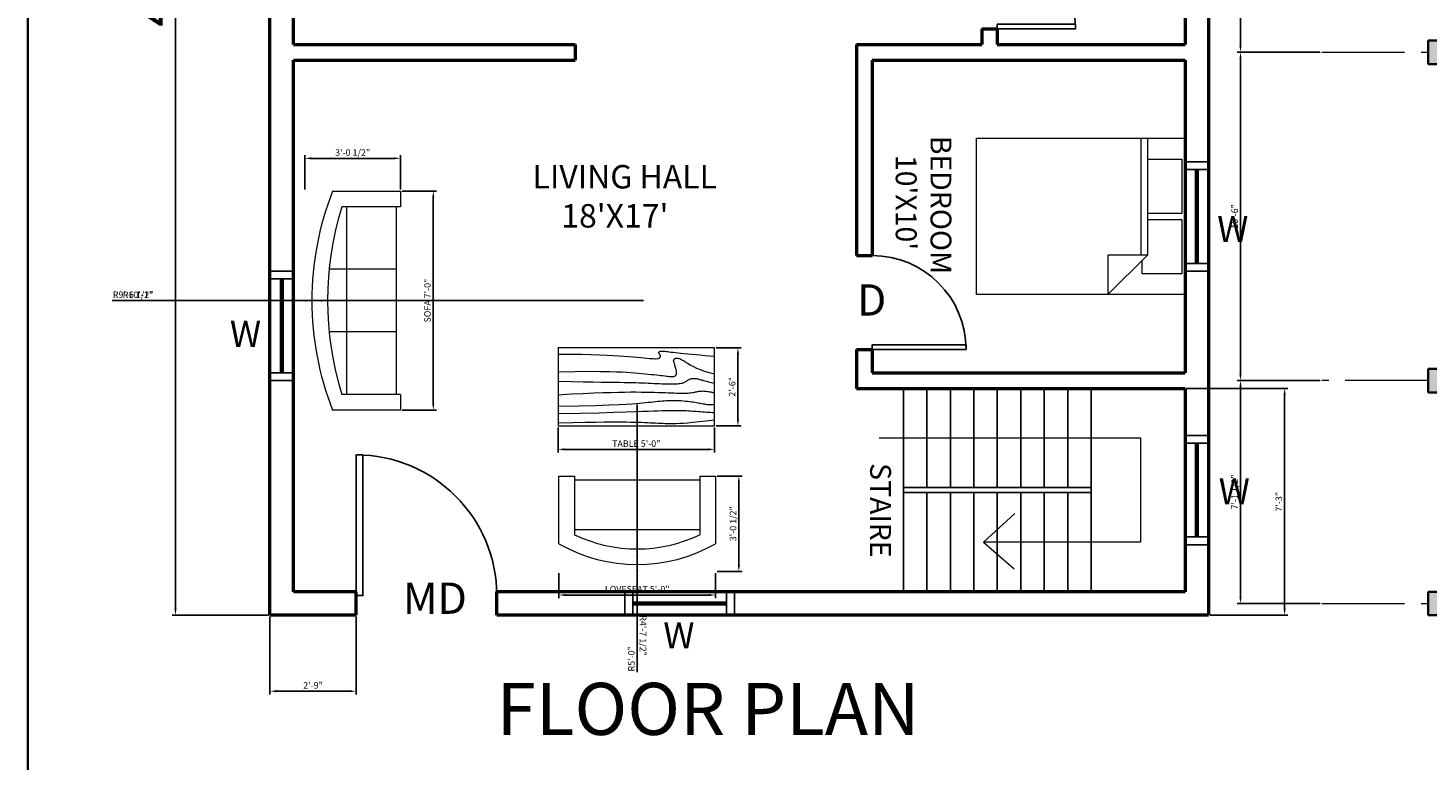
# Model space of a CAD drawing. Units: inches. Extents: x 2150 to 10686, y 1035 to 5077.
# Tile 2 of 12: x 2150 to 2687, y 1472 to 1753. Entities that reach past the tile are written whole.
import ezdxf

# ---------------------------------------------------------------- set-up
doc = ezdxf.new("R2010")
doc.units = ezdxf.units.IN
doc.linetypes.add('CENTER', pattern=[50.8, 31.75, -6.35, 6.35, -6.35])
for name, color, linetype, lineweight in [('A-ANNO-DIMS', 2, 'Continuous', 18), ('A-ANNO-IDEN', 2, 'Continuous', 18), ('A-ANNO-SYMB', 3, 'Continuous', 18), ('A-ANNO-TITL', 3, 'Continuous', 35), ('A-ANNO-TTLB', 7, 'Continuous', 35), ('A-AREA-IDEN', 7, 'Continuous', 18), ('A-COLS', 7, 'Continuous', 35), ('A-COLS-PATT', 8, 'Continuous', 13), ('A-DOOR', 4, 'Continuous', 25), ('A-FLOR-STRS', 4, 'Continuous', 25), ('A-FURN', 8, 'Continuous', 18), ('A-GLAZ', 30, 'Continuous', 25), ('A-GRID', 1, 'CENTER', 18), ('A-WALL', 18, 'Continuous', 50)]:
    doc.layers.add(name, color=color, linetype=linetype, lineweight=lineweight)
doc.styles.get("Standard").update_dxf_attribs({"font": 'arial.ttf'})
doc.dimstyles.new('ISO-25', dxfattribs={"dimtxt": 2.5, "dimasz": 2.5, "dimexe": 1.25, "dimexo": 0.625, "dimtad": 1, "dimdec": 0, "dimlunit": 3, "dimtxsty": 'Standard', "dimcen": 2.5, "dimadec": 0, "dimazin": 0, "dimtfac": 1, "dimtdec": 0, "dimtmove": 0, "dimatfit": 3, "dimfxl": 1, "dimarcsym": 0})

# ---------------------------------------------------------------- blocks, each defined once
blk = doc.blocks.new('Bed - Queen')
for p, q in [((0, -80.00003), (0, 0)), ((0, 0), (59.99999, 0)), ((59.99999, 0), (59.99999, -80.00003)), ((7.99999, -1.2), (28.79998, -1.2)), ((7.99999, -14.4), (7.99999, -1.2)), ((28.79998, -1.2), (28.79998, -14.4)), ((31.19999, -1.2), (51.99999, -1.2)), ((31.19999, -14.4), (31.19999, -1.2)), ((51.99999, -1.2), (51.99999, -16.4)), ((0, -14.4), (44.8, -14.4)), ((59.99999, -29.6), (44.8, -14.4)), ((44.8, -14.4), (44.8, -29.6)), ((44.8, -16.8), (0, -16.8)), ((51.99999, -16.4), (46.79936, -16.4)), ((44.8, -29.6), (59.99999, -29.6)), ((59.99999, -80.00003), (0, -80.00003))]:
    blk.add_line(p, q)
blk = doc.blocks.new('Sofa - Roundback 7 ft.')
for p, q in [((-12.00002, -32.4421), (-12.00003, -6.5971)), ((11.99997, -32.4421), (11.99998, -6.5971)), ((-36.000027, -34), (-36.000027, -11.4696)), ((-35.999844, -13.3819), (35.9998, -13.3819)), ((35.99998, -34), (35.99998, -11.4696)), ((-36.000027, -32.4421), (35.99998, -32.4421))]:
    blk.add_line(p, q)
for points in [[(-36.000027, -34), (-42.000027, -34), (-42.000027, -8)], [(41.99998, -8), (41.99998, -34), (35.99998, -34)]]:
    blk.add_lwpolyline(points)
for centre, radius, start, end in [((0, -114.25), 114.25, 68.43141, 111.5686), ((-0.00001, -127.1968), 121.1968, 72.72033, 107.2797)]:
    blk.add_arc(centre, radius, start, end)
blk = doc.blocks.new('Sofa - Roundback Loveseat 5 ft.')
for p, q in [((0, -32.44198), (0, -5.99998)), ((-24, -33.99998), (-24, -11.46958)), ((-23.9998, -13.38178), (23.99986, -13.38178)), ((24.00004, -33.99998), (24.00004, -11.46958)), ((-24, -32.44198), (24.00004, -32.44198))]:
    blk.add_line(p, q)
for points in [[(-24, -33.99998), (-30, -33.99998), (-30, -7.99998)], [(30.00004, -7.99998), (30.00004, -33.99998), (24.00004, -33.99998)]]:
    blk.add_lwpolyline(points)
for centre, radius, start, end in [((0, -60.24998), 60.24998, 60.13715, 119.8628), ((0, -61.38438), 55.38444, 64.32083, 115.6792)]:
    blk.add_arc(centre, radius, start, end)
blk = doc.blocks.new('Table - Rectangular Woodgrain 60 x 30 in.')
for p, q in [((0, 0), (0, -30)), ((60, 0), (0, 0)), ((60, -30), (60, 0)), ((0, -30), (60, -30))]:
    blk.add_line(p, q)
for points in [[(0, -2.4), (4.8155, -2.418), (9.0302, -2.4688), (12.709, -2.5477), (15.9167, -2.65), (18.7181, -2.7711), (21.1781, -2.9063), (23.3616, -3.0508), (25.3333, -3.2), (27.1477, -3.3495), (28.8172, -3.4958), (30.3437, -3.636), (31.7291, -3.7667), (32.9756, -3.8849), (34.0849, -3.9875), (35.059, -4.0714), (35.9, -4.1334), (36.6114, -4.1711), (37.2041, -4.1854), (37.6906, -4.1779), (38.0833, -4.15), (38.3948, -4.1034), (38.6375, -4.0396), (38.8239, -3.9602), (38.9666, -3.8667), (39.0764, -3.7608), (39.1573, -3.6448), (39.2116, -3.521), (39.2416, -3.3917), (39.2498, -3.2593), (39.2385, -3.1261), (39.21, -2.9944), (39.1666, -2.8667), (39.111, -2.7447), (39.0468, -2.6281), (38.978, -2.5163), (38.9083, -2.4083), (38.8418, -2.3035), (38.7823, -2.201), (38.7337, -2.1001), (38.7, -2), (38.6844, -1.9003), (38.6875, -1.8021), (38.7094, -1.707), (38.75, -1.6167), (38.8094, -1.5326), (38.8875, -1.4563), (38.9844, -1.3893), (39.1, -1.3333), (39.2351, -1.2896), (39.3937, -1.2583), (39.5804, -1.2396), (39.8, -1.2333), (40.057, -1.2396), (40.3562, -1.2583), (40.7023, -1.2896), (41.1, -1.3333), (41.5547, -1.3895), (42.0755, -1.4573), (42.6721, -1.5361), (43.3542, -1.625), (44.1316, -1.7233), (45.014, -1.8302), (46.0114, -1.9449), (47.1333, -2.0667), (48.3862, -2.1947), (49.7625, -2.3281), (51.2513, -2.4663), (52.8416, -2.6083), (54.5226, -2.7535), (56.2833, -2.9011), (58.1127, -3.0501), (60, -3.2)], [(0, -9.2), (6.5759, -9.0858), (11.9385, -9.0365), (16.2527, -9.0418), (19.6833, -9.0917), (22.3952, -9.1759), (24.5531, -9.2844), (26.322, -9.4069), (27.8666, -9.5333), (29.3241, -9.6553), (30.7203, -9.7719), (32.0532, -9.8837), (33.3208, -9.9917), (34.5213, -10.0965), (35.6526, -10.199), (36.7128, -10.2999), (37.7, -10.4), (38.6129, -10.4996), (39.4531, -10.5969), (40.223, -10.6895), (40.925, -10.775), (41.5613, -10.8512), (42.1344, -10.9156), (42.6465, -10.966), (43.1, -11), (43.4976, -11.0158), (43.8437, -11.0136), (44.143, -10.9942), (44.4, -10.9583), (44.6195, -10.9069), (44.8062, -10.8406), (44.9648, -10.7603), (45.1, -10.6667), (45.2155, -10.5598), (45.3114, -10.4365), (45.3871, -10.2929), (45.4416, -10.125), (45.4743, -9.929), (45.4844, -9.7011), (45.4709, -9.4371), (45.4333, -9.1333), (45.3716, -8.7883), (45.2896, -8.4104), (45.1919, -8.0107), (45.0833, -7.6), (44.9685, -7.1893), (44.8521, -6.7896), (44.7388, -6.4117), (44.6333, -6.0667), (44.54, -5.7628), (44.4614, -5.4979), (44.4001, -5.2675), (44.3583, -5.0667), (44.3384, -4.8909), (44.3427, -4.7354), (44.3736, -4.5956), (44.4333, -4.4667), (44.5236, -4.3453), (44.6427, -4.2333), (44.7884, -4.1339), (44.9583, -4.05), (45.1501, -3.9849), (45.3614, -3.9417), (45.59, -3.9234), (45.8333, -3.9333), (46.0915, -3.9749), (46.3734, -4.0531), (46.6906, -4.1736), (47.0542, -4.3417), (47.4756, -4.5629), (47.9661, -4.8427), (48.5372, -5.1866), (49.2, -5.6), (49.9676, -6.0844), (50.8594, -6.625), (51.8965, -7.2031), (53.1, -7.8), (54.491, -8.3969), (56.0906, -8.975), (57.9199, -9.5156), (60, -10)], [(0, -12.8), (5.1847, -12.9322), (9.6213, -13.0323), (13.3963, -13.1059), (16.5958, -13.1583), (19.3063, -13.1952), (21.614, -13.2219), (23.6054, -13.2439), (25.3666, -13.2667), (26.9728, -13.2947), (28.4531, -13.3281), (29.8256, -13.3663), (31.1083, -13.4083), (32.3191, -13.4535), (33.476, -13.501), (34.597, -13.5501), (35.7, -13.6), (36.7984, -13.6497), (37.8875, -13.6979), (38.9578, -13.743), (40, -13.7833), (41.0047, -13.8174), (41.9625, -13.8438), (42.864, -13.8607), (43.7, -13.8667), (44.4631, -13.8604), (45.1552, -13.8417), (45.7801, -13.8104), (46.3416, -13.7667), (46.8439, -13.7104), (47.2906, -13.6417), (47.6858, -13.5604), (48.0333, -13.4667), (48.3375, -13.3608), (48.6042, -13.2448), (48.8396, -13.121), (49.05, -12.9917), (49.2417, -12.8593), (49.4208, -12.7261), (49.5937, -12.5944), (49.7667, -12.4667), (49.9452, -12.3451), (50.1323, -12.2313), (50.3303, -12.1268), (50.5416, -12.0333), (50.7686, -11.9524), (51.0135, -11.8854), (51.2788, -11.8341), (51.5666, -11.8), (51.8785, -11.7843), (52.2116, -11.7865), (52.562, -11.8059), (52.926, -11.8417), (53.2998, -11.8931), (53.6795, -11.9594), (54.0614, -12.0397), (54.4416, -12.1333), (54.8223, -12.2401), (55.2293, -12.3625), (55.6942, -12.5037), (56.2489, -12.6667), (56.9251, -12.8547), (57.7545, -13.0708), (58.7689, -13.3182), (60, -13.6)], [(0, -18), (5.124, -17.7273), (9.6609, -17.5057), (13.6705, -17.3303), (17.2125, -17.1958), (20.3467, -17.0973), (23.1328, -17.0297), (25.6307, -16.9878), (27.9, -16.9667), (29.9928, -16.9617), (31.9302, -16.9703), (33.7254, -16.9907), (35.3917, -17.0208), (36.9423, -17.0588), (38.3906, -17.1026), (39.7499, -17.1503), (41.0333, -17.2), (42.2519, -17.2496), (43.4073, -17.2969), (44.4986, -17.3395), (45.525, -17.375), (46.4858, -17.4012), (47.3802, -17.4156), (48.2074, -17.416), (48.9667, -17.4), (49.6583, -17.3662), (50.2872, -17.3167), (50.8595, -17.2547), (51.3812, -17.1833), (51.8584, -17.1057), (52.2971, -17.025), (52.7034, -16.9443), (53.0833, -16.8667), (53.443, -16.7951), (53.789, -16.7313), (54.128, -16.6768), (54.4666, -16.6334), (54.8115, -16.6024), (55.1693, -16.5854), (55.5465, -16.5841), (55.95, -16.6), (56.3828, -16.6337), (56.8346, -16.6823), (57.2915, -16.7418), (57.7396, -16.8084), (58.165, -16.878), (58.5539, -16.9469), (58.8924, -17.0111), (59.1666, -17.0667), (59.3679, -17.1107), (59.5078, -17.1438), (59.6032, -17.1675), (59.6708, -17.1833), (59.7275, -17.193), (59.7901, -17.1979), (59.8753, -17.1998), (60, -17.2)], [(0, -22.4), (8.0098, -22.2501), (14.4094, -22.1011), (19.4168, -21.9535), (23.25, -21.8083), (26.1269, -21.6663), (28.2656, -21.5281), (29.884, -21.3947), (31.2, -21.2667), (32.3967, -21.1448), (33.5172, -21.0292), (34.5697, -20.9198), (35.5625, -20.8167), (36.5037, -20.7198), (37.4015, -20.6292), (38.2642, -20.5448), (39.1, -20.4667), (39.9164, -20.3951), (40.7187, -20.3313), (41.5117, -20.2768), (42.3, -20.2333), (43.0883, -20.2024), (43.8812, -20.1854), (44.6836, -20.1841), (45.5, -20.2), (46.3328, -20.234), (47.1747, -20.2844), (48.0163, -20.3488), (48.8479, -20.425), (49.66, -20.5106), (50.4429, -20.6031), (51.1872, -20.7004), (51.8833, -20.8), (52.5246, -20.8999), (53.1166, -20.9995), (53.6681, -21.0983), (54.1875, -21.1958), (54.6834, -21.2919), (55.1646, -21.3859), (55.6394, -21.4777), (56.1167, -21.5667), (56.6028, -21.6515), (57.0961, -21.7266), (57.5929, -21.7852), (58.0896, -21.8208), (58.5823, -21.8268), (59.0674, -21.7964), (59.5412, -21.723), (60, -21.6)], [(0, -25.2), (8.6355, -25.0504), (15.7026, -24.9031), (21.4049, -24.7606), (25.9458, -24.625), (29.529, -24.4988), (32.3578, -24.3844), (34.6359, -24.284), (36.5667, -24.2), (38.3213, -24.1341), (39.9417, -24.0854), (41.437, -24.0523), (42.8167, -24.0333), (44.0901, -24.0268), (45.2667, -24.0313), (46.3557, -24.0451), (47.3667, -24.0667), (48.309, -24.0947), (49.1928, -24.1287), (50.0284, -24.168), (50.826, -24.2125), (51.5959, -24.2617), (52.3483, -24.3151), (53.0935, -24.3725), (53.8417, -24.4334), (54.6009, -24.497), (55.3699, -24.561), (56.1454, -24.6226), (56.9239, -24.6792), (57.7021, -24.7279), (58.4764, -24.7662), (59.2435, -24.7911), (60, -24.8)], [(0, -28.8), (5.6867, -28.6681), (10.45, -28.5698), (14.407, -28.5012), (17.675, -28.4584), (20.3711, -28.4374), (22.6125, -28.4344), (24.5164, -28.4455), (26.2, -28.4667), (27.762, -28.4947), (29.2276, -28.5281), (30.6033, -28.5663), (31.8958, -28.6084), (33.1118, -28.6535), (34.2578, -28.7011), (35.3405, -28.7501), (36.3666, -28.8), (37.3443, -28.8497), (38.288, -28.8974), (39.2137, -28.9412), (40.1375, -28.9792), (41.0753, -29.0093), (42.0432, -29.0297), (43.0572, -29.0384), (44.1333, -29.0333), (45.2936, -29.0114), (46.5843, -28.9641), (48.0579, -28.8816), (49.7666, -28.7542), (51.7629, -28.5721), (54.0989, -28.3255), (56.8272, -28.0048), (60, -27.6)]]:
    blk.add_lwpolyline(points)
blk = doc.blocks.new('*U9')
for p, q in [((0, 0), (0, -6)), ((-36, 0), (-36, -6))]:
    blk.add_line(p, q)
blk.add_lwpolyline([(0, 0), (0, 36), (-1.75, 36), (-1.75, 0)], close=True)
blk.add_arc((0, 0), 36, 90, 180)
blk = doc.blocks.new('*U10')
for p, q in [((-30, 0), (-30, -6)), ((0, 0), (0, -6))]:
    blk.add_line(p, q)
blk.add_lwpolyline([(0, 0), (0, 30), (-1.75, 30), (-1.75, 0)], close=True)
blk.add_arc((0, 0), 30, 90, 180)
blk = doc.blocks.new('*U11')
for p, q in [((0, 0), (0, -5)), ((36, 0), (36, -5))]:
    blk.add_line(p, q)
blk.add_lwpolyline([(0, 0), (0, 36), (1.75, 36), (1.75, 0)], close=True)
blk.add_arc((0, 0), 36, 0, 90)
blk = doc.blocks.new('*D13')
at = {"layer": 'A-ANNO-DIMS', "color": 0, "lineweight": -2, "transparency": 16777216}
for p, q in [((2242.07, 2007.29), (2205.18, 2007.29)), ((2206.43, 2004.79), (2206.43, 1529.79)), ((2242.07, 1527.29), (2205.18, 1527.29))]:
    blk.add_line(p, q, dxfattribs=at)
at = {"layer": 'A-ANNO-DIMS', "color": 0, "transparency": 16777216}
for points in [[(2206.01, 2004.79), (2206.85, 2004.79), (2206.43, 2007.29)], [(2206.01, 1529.79), (2206.85, 1529.79), (2206.43, 1527.29)]]:
    blk.add_solid(points, dxfattribs=at)
at = {"layer": 'Defpoints', "color": 0, "transparency": 16777216}
for p in [(2242.69, 2007.29), (2206.43, 1527.29), (2242.69, 1527.29)]:
    blk.add_point(p, dxfattribs=at)
at = {"layer": 'A-ANNO-DIMS', "color": 0, "transparency": 16777216, "insert": (2198.15, 1767.29), "char_height": 2.5, "attachment_point": 5, "rotation": 90}
blk.add_mtext("{\\H6x;40'}", dxfattribs=at)
blk = doc.blocks.new('COL-SQUARE-9IN')
for p, q in [((0, 9), (9, 9)), ((0, 0), (0, 9)), ((9, 9), (9, 0)), ((9, 0), (0, 0))]:
    blk.add_line(p, q)
blk = doc.blocks.new('WINDOW-36IN')
for p, q in [((9, 42), (0, 42)), ((9, 39), (0, 39)), ((4, 39), (4, 3)), ((4.5, 39), (4.5, 3)), ((5, 39), (5, 3)), ((9, 3), (0, 3)), ((9, 0), (0, 0))]:
    blk.add_line(p, q)
blk = doc.blocks.new('*D48')
at = {"layer": 'A-ANNO-DIMS', "color": 0, "lineweight": -2, "transparency": 16777216}
for p, q in [((2293.35, 1690), (2306.58, 1690)), ((2305.33, 1608.5), (2305.33, 1687.5)), ((2293.35, 1606), (2306.58, 1606))]:
    blk.add_line(p, q, dxfattribs=at)
at = {"layer": 'A-ANNO-DIMS', "color": 0, "transparency": 16777216}
for points in [[(2304.91, 1687.5), (2305.75, 1687.5), (2305.33, 1690)], [(2304.91, 1608.5), (2305.75, 1608.5), (2305.33, 1606)]]:
    blk.add_solid(points, dxfattribs=at)
at = {"layer": 'Defpoints', "color": 0, "transparency": 16777216}
for p in [(2292.73, 1690), (2305.33, 1690), (2292.73, 1606)]:
    blk.add_point(p, dxfattribs=at)
at = {"layer": 'A-ANNO-DIMS', "color": 0, "transparency": 16777216, "insert": (2303.41, 1648), "char_height": 2.5, "attachment_point": 5, "rotation": 90}
blk.add_mtext('SOFA 7\'-0"', dxfattribs=at)
blk = doc.blocks.new('*D49')
at = {"layer": 'A-ANNO-DIMS', "color": 0, "lineweight": -2, "transparency": 16777216}
for p, q in [((2256.06, 1690.62), (2256.06, 1703.85)), ((2290.23, 1702.6), (2258.56, 1702.6)), ((2292.73, 1690.62), (2292.73, 1703.85))]:
    blk.add_line(p, q, dxfattribs=at)
at = {"layer": 'A-ANNO-DIMS', "color": 0, "transparency": 16777216}
for points in [[(2258.56, 1703.01), (2258.56, 1702.18), (2256.06, 1702.6)], [(2290.23, 1703.01), (2290.23, 1702.18), (2292.73, 1702.6)]]:
    blk.add_solid(points, dxfattribs=at)
at = {"layer": 'Defpoints', "color": 0, "transparency": 16777216}
for p in [(2256.06, 1702.6), (2256.06, 1690), (2292.73, 1690)]:
    blk.add_point(p, dxfattribs=at)
at = {"layer": 'A-ANNO-DIMS', "color": 0, "transparency": 16777216, "insert": (2274.4, 1704.52), "char_height": 2.5, "attachment_point": 5}
blk.add_mtext('3\'-0 1/2"', dxfattribs=at)
blk = doc.blocks.new('*D52')
at = {"layer": 'A-ANNO-DIMS', "color": 0, "lineweight": -2, "transparency": 16777216}
for p, q in [((2353.54, 1543.39), (2353.54, 1533.76)), ((2413.54, 1543.39), (2413.54, 1533.76)), ((2411.04, 1535.01), (2356.04, 1535.01))]:
    blk.add_line(p, q, dxfattribs=at)
at = {"layer": 'A-ANNO-DIMS', "color": 0, "transparency": 16777216}
for points in [[(2356.04, 1535.43), (2356.04, 1534.6), (2353.54, 1535.01)], [(2411.04, 1535.43), (2411.04, 1534.6), (2413.54, 1535.01)]]:
    blk.add_solid(points, dxfattribs=at)
at = {"layer": 'Defpoints', "color": 0, "transparency": 16777216}
for p in [(2353.54, 1544.01), (2413.54, 1544.01), (2353.54, 1535.01)]:
    blk.add_point(p, dxfattribs=at)
at = {"layer": 'A-ANNO-DIMS', "color": 0, "transparency": 16777216, "insert": (2383.54, 1536.93), "char_height": 2.5, "attachment_point": 5}
blk.add_mtext('LOVESEAT 5\'-0"', dxfattribs=at)
blk = doc.blocks.new('*D53')
at = {"layer": 'A-ANNO-DIMS', "color": 0, "lineweight": -2, "transparency": 16777216}
for p, q in [((2414.17, 1580.68), (2423.79, 1580.68)), ((2422.54, 1578.18), (2422.54, 1546.51)), ((2414.17, 1544.01), (2423.79, 1544.01))]:
    blk.add_line(p, q, dxfattribs=at)
at = {"layer": 'A-ANNO-DIMS', "color": 0, "transparency": 16777216}
for points in [[(2422.13, 1578.18), (2422.96, 1578.18), (2422.54, 1580.68)], [(2422.13, 1546.51), (2422.96, 1546.51), (2422.54, 1544.01)]]:
    blk.add_solid(points, dxfattribs=at)
at = {"layer": 'Defpoints', "color": 0, "transparency": 16777216}
for p in [(2413.54, 1580.68), (2413.54, 1544.01), (2422.54, 1544.01)]:
    blk.add_point(p, dxfattribs=at)
at = {"layer": 'A-ANNO-DIMS', "color": 0, "transparency": 16777216, "insert": (2420.63, 1562.35), "char_height": 2.5, "attachment_point": 5, "rotation": 90}
blk.add_mtext('3\'-0 1/2"', dxfattribs=at)
blk = doc.blocks.new('*D60')
at = {"layer": 'A-ANNO-DIMS', "color": 0, "lineweight": -2, "transparency": 16777216}
for p, q in [((2353.19, 1599.26), (2353.19, 1589.64)), ((2413.19, 1599.26), (2413.19, 1589.64)), ((2355.69, 1590.89), (2410.69, 1590.89))]:
    blk.add_line(p, q, dxfattribs=at)
at = {"layer": 'A-ANNO-DIMS', "color": 0, "transparency": 16777216}
for points in [[(2355.69, 1591.31), (2355.69, 1590.47), (2353.19, 1590.89)], [(2410.69, 1591.31), (2410.69, 1590.47), (2413.19, 1590.89)]]:
    blk.add_solid(points, dxfattribs=at)
at = {"layer": 'Defpoints', "color": 0, "transparency": 16777216}
for p in [(2353.19, 1599.89), (2413.19, 1599.89), (2413.19, 1590.89)]:
    blk.add_point(p, dxfattribs=at)
at = {"layer": 'A-ANNO-DIMS', "color": 0, "transparency": 16777216, "insert": (2383.19, 1592.79), "char_height": 2.5, "attachment_point": 5}
blk.add_mtext('TABLE 5\'-0"', dxfattribs=at)
blk = doc.blocks.new('*D61')
at = {"layer": 'A-ANNO-DIMS', "color": 0, "lineweight": -2, "transparency": 16777216}
for p, q in [((2413.81, 1629.89), (2423.44, 1629.89)), ((2422.19, 1602.39), (2422.19, 1627.39)), ((2413.81, 1599.89), (2423.44, 1599.89))]:
    blk.add_line(p, q, dxfattribs=at)
at = {"layer": 'A-ANNO-DIMS', "color": 0, "transparency": 16777216}
for points in [[(2421.77, 1627.39), (2422.6, 1627.39), (2422.19, 1629.89)], [(2421.77, 1602.39), (2422.6, 1602.39), (2422.19, 1599.89)]]:
    blk.add_solid(points, dxfattribs=at)
at = {"layer": 'Defpoints', "color": 0, "transparency": 16777216}
for p in [(2413.19, 1629.89), (2422.19, 1629.89), (2413.19, 1599.89)]:
    blk.add_point(p, dxfattribs=at)
at = {"layer": 'A-ANNO-DIMS', "color": 0, "transparency": 16777216, "insert": (2420.29, 1614.89), "char_height": 2.5, "attachment_point": 5, "rotation": 90}
blk.add_mtext('2\'-6"', dxfattribs=at)
blk = doc.blocks.new('*D81')
at = {"layer": 'A-ANNO-DIMS', "color": 0, "lineweight": -2, "transparency": 16777216}
for p, q in [((2645.54, 1869.29), (2613.71, 1869.29)), ((2614.96, 1866.79), (2614.96, 1745.79)), ((2645.54, 1743.29), (2613.71, 1743.29))]:
    blk.add_line(p, q, dxfattribs=at)
at = {"layer": 'A-ANNO-DIMS', "color": 0, "transparency": 16777216}
for points in [[(2614.55, 1866.79), (2615.38, 1866.79), (2614.96, 1869.29)], [(2614.55, 1745.79), (2615.38, 1745.79), (2614.96, 1743.29)]]:
    blk.add_solid(points, dxfattribs=at)
at = {"layer": 'Defpoints', "color": 0, "transparency": 16777216}
for p in [(2646.16, 1869.29), (2614.96, 1743.29), (2646.16, 1743.29)]:
    blk.add_point(p, dxfattribs=at)
at = {"layer": 'A-ANNO-DIMS', "color": 0, "transparency": 16777216, "insert": (2613.06, 1806.29), "char_height": 2.5, "attachment_point": 5, "rotation": 90}
blk.add_mtext('10\'-6"', dxfattribs=at)
blk = doc.blocks.new('*D82')
at = {"layer": 'A-ANNO-DIMS', "color": 0, "lineweight": -2, "transparency": 16777216}
for p, q in [((2645.54, 1743.29), (2613.71, 1743.29)), ((2614.96, 1740.79), (2614.96, 1619.79)), ((2645.54, 1617.29), (2613.71, 1617.29))]:
    blk.add_line(p, q, dxfattribs=at)
at = {"layer": 'A-ANNO-DIMS', "color": 0, "transparency": 16777216}
for points in [[(2614.55, 1740.79), (2615.38, 1740.79), (2614.96, 1743.29)], [(2614.55, 1619.79), (2615.38, 1619.79), (2614.96, 1617.29)]]:
    blk.add_solid(points, dxfattribs=at)
at = {"layer": 'Defpoints', "color": 0, "transparency": 16777216}
for p in [(2646.16, 1743.29), (2614.96, 1617.29), (2646.16, 1617.29)]:
    blk.add_point(p, dxfattribs=at)
at = {"layer": 'A-ANNO-DIMS', "color": 0, "transparency": 16777216, "insert": (2613.06, 1680.29), "char_height": 2.5, "attachment_point": 5, "rotation": 90}
blk.add_mtext('10\'-6"', dxfattribs=at)
blk = doc.blocks.new('*D83')
at = {"layer": 'A-ANNO-DIMS', "color": 0, "lineweight": -2, "transparency": 16777216}
for p, q in [((2645.54, 1617.29), (2613.71, 1617.29)), ((2614.96, 1614.79), (2614.96, 1534.29)), ((2645.54, 1531.79), (2613.71, 1531.79))]:
    blk.add_line(p, q, dxfattribs=at)
at = {"layer": 'A-ANNO-DIMS', "color": 0, "transparency": 16777216}
for points in [[(2614.55, 1614.79), (2615.38, 1614.79), (2614.96, 1617.29)], [(2614.55, 1534.29), (2615.38, 1534.29), (2614.96, 1531.79)]]:
    blk.add_solid(points, dxfattribs=at)
at = {"layer": 'Defpoints', "color": 0, "transparency": 16777216}
for p in [(2646.16, 1617.29), (2614.96, 1531.79), (2646.16, 1531.79)]:
    blk.add_point(p, dxfattribs=at)
at = {"layer": 'A-ANNO-DIMS', "color": 0, "transparency": 16777216, "insert": (2613.05, 1574.54), "char_height": 2.5, "attachment_point": 5, "rotation": 90}
blk.add_mtext('7\'-1 1/2"', dxfattribs=at)
blk = doc.blocks.new('*D139')
at = {"layer": 'A-ANNO-DIMS', "color": 0, "lineweight": -2, "transparency": 16777216}
for p, q in [((2242.69, 1526.67), (2242.69, 1496.84)), ((2275.69, 1526.67), (2275.69, 1496.84)), ((2245.19, 1498.09), (2273.19, 1498.09))]:
    blk.add_line(p, q, dxfattribs=at)
at = {"layer": 'A-ANNO-DIMS', "color": 0, "transparency": 16777216}
for points in [[(2245.19, 1498.51), (2245.19, 1497.67), (2242.69, 1498.09)], [(2273.19, 1498.51), (2273.19, 1497.67), (2275.69, 1498.09)]]:
    blk.add_solid(points, dxfattribs=at)
at = {"layer": 'Defpoints', "color": 0, "transparency": 16777216}
for p in [(2242.69, 1527.29), (2275.69, 1527.29), (2275.69, 1498.09)]:
    blk.add_point(p, dxfattribs=at)
at = {"layer": 'A-ANNO-DIMS', "color": 0, "transparency": 16777216, "insert": (2259.19, 1499.99), "char_height": 2.5, "attachment_point": 5}
blk.add_mtext('2\'-9"', dxfattribs=at)
blk = doc.blocks.new('*D140')
at = {"layer": 'A-ANNO-DIMS', "color": 0, "lineweight": -2, "transparency": 16777216}
for p, q in [((2594.32, 1614.29), (2633.14, 1614.29)), ((2631.89, 1529.79), (2631.89, 1611.79)), ((2603.32, 1527.29), (2633.14, 1527.29))]:
    blk.add_line(p, q, dxfattribs=at)
at = {"layer": 'A-ANNO-DIMS', "color": 0, "transparency": 16777216}
for points in [[(2631.48, 1611.79), (2632.31, 1611.79), (2631.89, 1614.29)], [(2631.48, 1529.79), (2632.31, 1529.79), (2631.89, 1527.29)]]:
    blk.add_solid(points, dxfattribs=at)
at = {"layer": 'Defpoints', "color": 0, "transparency": 16777216}
for p in [(2593.69, 1614.29), (2631.89, 1614.29), (2602.69, 1527.29)]:
    blk.add_point(p, dxfattribs=at)
at = {"layer": 'A-ANNO-DIMS', "color": 0, "transparency": 16777216, "insert": (2629.99, 1570.79), "char_height": 2.5, "attachment_point": 5, "rotation": 90}
blk.add_mtext('7\'-3"', dxfattribs=at)
blk = doc.blocks.new('*D147')
at = {"layer": 'A-ANNO-DIMS', "color": 0, "lineweight": -2, "transparency": 16777216}
for p, q in [((2185.9, 1648), (2262.23, 1648)), ((2385.93, 1648), (2264.73, 1648))]:
    blk.add_line(p, q, dxfattribs=at)
at = {"layer": 'A-ANNO-DIMS', "color": 0, "transparency": 16777216}
blk.add_solid([(2262.23, 1648.41), (2262.23, 1647.58), (2264.73, 1648)], dxfattribs=at)
at = {"layer": 'Defpoints', "color": 0, "transparency": 16777216}
for p in [(2264.73, 1648), (2385.93, 1648)]:
    blk.add_point(p, dxfattribs=at)
at = {"layer": 'A-ANNO-DIMS', "color": 0, "transparency": 16777216, "insert": (2192.01, 1649.9), "char_height": 2.5, "attachment_point": 5, "rotation": 0.0001}
blk.add_mtext('R10\'-1"', dxfattribs=at)
blk = doc.blocks.new('*D148')
at = {"layer": 'A-ANNO-DIMS', "color": 0, "lineweight": -2, "transparency": 16777216}
for p, q in [((2182.12, 1648), (2256.23, 1648)), ((2372.98, 1648), (2258.73, 1648))]:
    blk.add_line(p, q, dxfattribs=at)
at = {"layer": 'A-ANNO-DIMS', "color": 0, "transparency": 16777216}
blk.add_solid([(2256.23, 1648.41), (2256.23, 1647.58), (2258.73, 1648)], dxfattribs=at)
at = {"layer": 'Defpoints', "color": 0, "transparency": 16777216}
for p in [(2258.73, 1648), (2372.98, 1648)]:
    blk.add_point(p, dxfattribs=at)
at = {"layer": 'A-ANNO-DIMS', "color": 0, "transparency": 16777216, "insert": (2190.18, 1649.92), "char_height": 2.5, "attachment_point": 5, "rotation": 0.0001}
blk.add_mtext('R9\'-6 1/2"', dxfattribs=at)
blk = doc.blocks.new('*D149')
at = {"layer": 'A-ANNO-DIMS', "color": 0, "lineweight": -2, "transparency": 16777216}
for p, q in [((2383.54, 1606.93), (2383.54, 1546.68)), ((2383.54, 1505.39), (2383.54, 1544.18))]:
    blk.add_line(p, q, dxfattribs=at)
at = {"layer": 'A-ANNO-DIMS', "color": 0, "transparency": 16777216}
blk.add_solid([(2383.13, 1544.18), (2383.96, 1544.18), (2383.54, 1546.68)], dxfattribs=at)
at = {"layer": 'Defpoints', "color": 0, "transparency": 16777216}
for p in [(2383.54, 1606.93), (2383.54, 1546.68)]:
    blk.add_point(p, dxfattribs=at)
at = {"layer": 'A-ANNO-DIMS', "color": 0, "transparency": 16777216, "insert": (2381.64, 1510.53), "char_height": 2.5, "attachment_point": 5, "rotation": 89.9995}
blk.add_mtext('R5\'-0"', dxfattribs=at)
blk = doc.blocks.new('*D150')
at = {"layer": 'A-ANNO-DIMS', "color": 0, "lineweight": -2, "transparency": 16777216}
for p, q in [((2383.54, 1608.06), (2383.54, 1552.68)), ((2383.54, 1511.39), (2383.54, 1550.18))]:
    blk.add_line(p, q, dxfattribs=at)
at = {"layer": 'A-ANNO-DIMS', "color": 0, "transparency": 16777216}
blk.add_solid([(2383.96, 1550.18), (2383.13, 1550.18), (2383.54, 1552.68)], dxfattribs=at)
at = {"layer": 'Defpoints', "color": 0, "transparency": 16777216}
for p in [(2383.54, 1608.06), (2383.54, 1552.68)]:
    blk.add_point(p, dxfattribs=at)
at = {"layer": 'A-ANNO-DIMS', "color": 0, "transparency": 16777216, "insert": (2385.46, 1519.45), "char_height": 2.5, "attachment_point": 5, "rotation": 270.0005}
blk.add_mtext('R4\'-7 1/2"', dxfattribs=at)

msp = doc.modelspace()

# ---------------------------------------------------------------- hatches: boundary and pattern name
at = {"layer": 'A-COLS-PATT'}
h = msp.add_hatch(color=256, dxfattribs=at)
h.dxf.hatch_style = 1
h.paths.add_polyline_path([(2695.9, 2007.29), (2686.9, 2007.29), (2686.9, 1998.29), (2695.9, 1998.29)])
h.paths.add_polyline_path([(2871.4, 2007.29), (2862.4, 2007.29), (2862.4, 1998.29), (2871.4, 1998.29)])
h.paths.add_polyline_path([(3046.9, 2007.29), (3037.9, 2007.29), (3037.9, 1998.29), (3046.9, 1998.29)])
h.paths.add_polyline_path([(2695.9, 1873.79), (2686.9, 1873.79), (2686.9, 1864.79), (2695.9, 1864.79)])
h.paths.add_polyline_path([(2871.4, 1873.79), (2862.4, 1873.79), (2862.4, 1864.79), (2871.4, 1864.79)])
h.paths.add_polyline_path([(3046.9, 1873.79), (3037.9, 1873.79), (3037.9, 1864.79), (3046.9, 1864.79)])
h.paths.add_polyline_path([(2695.9, 1747.79), (2686.9, 1747.79), (2686.9, 1738.79), (2695.9, 1738.79)])
h.paths.add_polyline_path([(2871.4, 1747.79), (2862.4, 1747.79), (2862.4, 1738.79), (2871.4, 1738.79)])
h.paths.add_polyline_path([(3046.9, 1747.79), (3037.9, 1747.79), (3037.9, 1738.79), (3046.9, 1738.79)])
h.paths.add_polyline_path([(2695.9, 1621.79), (2686.9, 1621.79), (2686.9, 1612.79), (2695.9, 1612.79)])
h.paths.add_polyline_path([(2871.4, 1621.79), (2862.4, 1621.79), (2862.4, 1612.79), (2871.4, 1612.79)])
h.paths.add_polyline_path([(3046.9, 1621.79), (3037.9, 1621.79), (3037.9, 1612.79), (3046.9, 1612.79)])
h.paths.add_polyline_path([(2695.9, 1536.29), (2686.9, 1536.29), (2686.9, 1527.29), (2695.9, 1527.29)])
h.paths.add_polyline_path([(2871.4, 1536.29), (2862.4, 1536.29), (2862.4, 1527.29), (2871.4, 1527.29)])
h.paths.add_polyline_path([(3046.9, 1536.29), (3037.9, 1536.29), (3037.9, 1527.29), (3046.9, 1527.29)])

# ---------------------------------------------------------------- linework, layer by layer
at = {"layer": 'A-ANNO-SYMB'}
for p, q in [((2476.32, 1595.29), (2576.67, 1595.29)), ((2576.67, 1595.29), (2576.67, 1555.29)), ((2516.33, 1555.29), (2528.47, 1566.24)), ((2576.67, 1555.29), (2516.33, 1555.29)), ((2516.33, 1555.29), (2528.11, 1545.03))]:
    msp.add_line(p, q, dxfattribs=at)
at = {"layer": 'A-ANNO-TTLB'}
msp.add_lwpolyline([(2149.86, 2100.72), (3159.01, 2100.72), (3159.01, 1034.91), (2149.86, 1034.91)], close=True, dxfattribs=at)
at = {"layer": 'A-FLOR-STRS'}
for p, q in [((2485.69, 1614.29), (2485.69, 1536.29)), ((2494.69, 1614.29), (2494.69, 1576.29)), ((2503.69, 1614.29), (2503.69, 1576.29)), ((2512.69, 1614.29), (2512.69, 1576.29)), ((2521.69, 1614.29), (2521.69, 1576.29)), ((2530.69, 1614.29), (2530.69, 1576.29)), ((2539.69, 1614.29), (2539.69, 1576.29)), ((2548.69, 1614.29), (2548.69, 1576.29)), ((2557.69, 1614.29), (2557.69, 1536.29)), ((2557.69, 1576.29), (2485.69, 1576.29)), ((2557.69, 1574.29), (2485.69, 1574.29)), ((2494.69, 1574.29), (2494.69, 1536.29)), ((2503.69, 1574.29), (2503.69, 1536.29)), ((2512.69, 1574.29), (2512.69, 1536.29)), ((2521.69, 1574.29), (2521.69, 1536.29)), ((2530.69, 1574.29), (2530.69, 1536.29)), ((2539.69, 1574.29), (2539.69, 1536.29)), ((2548.69, 1574.29), (2548.69, 1536.29))]:
    msp.add_line(p, q, dxfattribs=at)
at = {"layer": 'A-GRID'}
for p, q in [((2646.16, 1743.29), (2686.9, 1743.29)), ((2686.9, 1617.29), (2646.16, 1617.29)), ((2646.16, 1531.79), (2686.9, 1531.79))]:
    msp.add_line(p, q, dxfattribs=at)
at = {"layer": 'A-WALL'}
for p, q in [((2242.69, 1527.29), (2242.69, 2007.29)), ((2602.69, 2007.29), (2602.69, 1527.29)), ((2251.69, 1746.29), (2251.69, 1866.29)), ((2593.69, 1818.29), (2593.69, 1746.29)), ((2515.69, 1752.29), (2521.69, 1752.29)), ((2515.69, 1752.29), (2515.69, 1746.29)), ((2521.69, 1752.29), (2521.69, 1746.29)), ((2251.69, 1746.29), (2359.69, 1746.29)), ((2359.69, 1746.29), (2359.69, 1740.29)), ((2467.69, 1746.29), (2515.69, 1746.29)), ((2467.69, 1746.29), (2467.69, 1665.29)), ((2521.69, 1746.29), (2593.69, 1746.29)), ((2251.69, 1536.29), (2251.69, 1740.29)), ((2251.69, 1740.29), (2359.69, 1740.29)), ((2473.69, 1740.29), (2593.69, 1740.29)), ((2473.69, 1740.29), (2473.69, 1665.29)), ((2593.69, 1740.29), (2593.69, 1620.29)), ((2467.69, 1665.29), (2473.69, 1665.29)), ((2467.69, 1629.29), (2473.69, 1629.29)), ((2467.69, 1629.29), (2467.69, 1614.29)), ((2473.69, 1629.29), (2473.69, 1620.29)), ((2473.69, 1620.29), (2593.69, 1620.29)), ((2467.69, 1614.29), (2593.69, 1614.29)), ((2593.69, 1614.29), (2593.69, 1536.29)), ((2275.69, 1536.29), (2251.69, 1536.29)), ((2275.69, 1527.29), (2275.69, 1536.29)), ((2593.69, 1536.29), (2329.69, 1536.29)), ((2329.69, 1527.29), (2329.69, 1536.29)), ((2275.69, 1527.29), (2242.69, 1527.29)), ((2602.69, 1527.29), (2329.69, 1527.29))]:
    msp.add_line(p, q, dxfattribs=at)

# ---------------------------------------------------------------- block references
at = {"layer": 'A-COLS'}
for p in [(2686.9, 1738.79), (2686.9, 1612.79), (2686.9, 1527.29)]:
    msp.add_blockref('COL-SQUARE-9IN', p, dxfattribs=at)
at = {"layer": 'A-DOOR', "rotation": 270}
for name, p in [('*U10', (2521.69, 1752.29)), ('*U9', (2473.69, 1629.29))]:
    msp.add_blockref(name, p, dxfattribs=at)
at = {"layer": 'A-DOOR', "xscale": 1.5, "yscale": 1.5, "zscale": 1.5}
msp.add_blockref('*U11', (2275.69, 1534.79), dxfattribs=at)
at = {"layer": 'A-FURN'}
for name, p, rotation in [('Bed - Queen', (2593.69, 1710.29), 270), ('Sofa - Roundback 7 ft.', (2258.73, 1648), 90), ('Sofa - Roundback Loveseat 5 ft.', (2383.54, 1546.68), 180)]:
    msp.add_blockref(name, p, dxfattribs=dict(at, rotation=rotation))
msp.add_blockref('Table - Rectangular Woodgrain 60 x 30 in.', (2353.19, 1629.89), dxfattribs=at)
at = {"layer": 'A-GLAZ'}
for p in [(2593.69, 1659.29), (2242.69, 1617.29)]:
    msp.add_blockref('WINDOW-36IN', p, dxfattribs=at)
for p, rotation in [((2602.69, 1596.29), 180), ((2420.82, 1527.29), 89.99999999999767)]:
    msp.add_blockref('WINDOW-36IN', p, dxfattribs=dict(at, rotation=rotation))

# ---------------------------------------------------------------- texts
at = {"layer": 'A-ANNO-IDEN', "attachment_point": 1}
for s, width, insert, char_height in [('W', 198.2229, (2606.02, 1680.44), 10), ('D', 907.773, (2467.84, 1654.25), 12), ('W', 198.2229, (2227.3, 1640.24), 10), ('W', 198.2229, (2606.6, 1579.8), 10), ('MD', 907.773, (2293.66, 1539.78), 12), ('W', 198.2229, (2393.55, 1524.53), 10)]:
    msp.add_mtext_dynamic_manual_height_columns(s, width=width, gutter_width=12.5, heights=[0], dxfattribs=dict(at, insert=insert, char_height=char_height))
at = {"layer": 'A-ANNO-TITL', "insert": (2329.62, 1501.3), "char_height": 20, "attachment_point": 1}
msp.add_mtext_dynamic_manual_height_columns('FLOOR PLAN', width=668.9491, gutter_width=12.5, heights=[0], dxfattribs=at)
at = {"layer": 'A-AREA-IDEN', "char_height": 8, "attachment_point": 1, "rotation": 270}
for s, width, insert in [("BEDROOM\\P   10'X10'", 364.331, (2504.07, 1711.25)), ('STAIRE', 364.1476, (2480.91, 1585.64))]:
    msp.add_mtext_dynamic_manual_height_columns(s, width=width, gutter_width=12.5, heights=[0], dxfattribs=dict(at, insert=insert))
at = {"layer": 'A-AREA-IDEN', "insert": (2343.42, 1700.03), "char_height": 9, "attachment_point": 1}
msp.add_mtext_dynamic_manual_height_columns("LIVING HALL\\P    18'X17'", width=702.7883, gutter_width=12.5, heights=[0], dxfattribs=at)

# ---------------------------------------------------------------- dimensions: what is measured, and where the dimension line sits
at = {"layer": 'A-ANNO-DIMS'}
for base, p1, p2, angle, text, override, picture, middle in [((2206.43, 1527.29), (2242.69, 2007.29), (2242.69, 1527.29), 90, '{\\H6x;<>}', {"dimclrd": 0, "dimclre": 0, "dimclrt": 0}, '*D13', (2198.15, 1767.29)), ((2305.33, 1690), (2292.73, 1606), (2292.73, 1690), 90, 'SOFA <>', {"dimdec": 1, "dimlfac": 1, "dimrnd": 0, "dimzin": 1, "dimdsep": 46, "dimlunit": 4, "dimfrac": 2}, '*D48', (2303.41, 1648)), ((2353.54, 1535.01), (2413.54, 1544.01), (2353.54, 1544.01), 180, 'LOVESEAT <>', {"dimdec": 1, "dimlfac": 1, "dimrnd": 0, "dimzin": 1, "dimdsep": 46, "dimlunit": 4, "dimfrac": 2}, '*D52', (2383.54, 1536.93))]:
    dim = msp.add_linear_dim(base=base, p1=p1, p2=p2, angle=angle, text=text, dimstyle='ISO-25', override=override, dxfattribs=at)
    dim.commit()
    dim.dimension.update_dxf_attribs({"geometry": picture, "text_midpoint": middle})
for base, p1, p2, angle, picture, middle in [((2614.96, 1743.29), (2646.16, 1869.29), (2646.16, 1743.29), 90, '*D81', (2613.06, 1806.29)), ((2614.96, 1617.29), (2646.16, 1743.29), (2646.16, 1617.29), 90, '*D82', (2613.06, 1680.29)), ((2256.06, 1702.6), (2292.73, 1690), (2256.06, 1690), 180, '*D49', (2274.4, 1704.52)), ((2422.19, 1629.89), (2413.19, 1599.89), (2413.19, 1629.89), 90, '*D61', (2420.29, 1614.89)), ((2614.96, 1531.79), (2646.16, 1617.29), (2646.16, 1531.79), 90, '*D83', (2613.05, 1574.54)), ((2631.89, 1614.29), (2602.69, 1527.29), (2593.69, 1614.29), 90, '*D140', (2629.99, 1570.79)), ((2422.54, 1544.01), (2413.54, 1580.68), (2413.54, 1544.01), 270, '*D53', (2420.63, 1562.35))]:
    dim = msp.add_linear_dim(base=base, p1=p1, p2=p2, angle=angle, dimstyle='ISO-25', override={"dimdec": 1, "dimlfac": 1, "dimrnd": 0, "dimzin": 1, "dimdsep": 46, "dimlunit": 4, "dimfrac": 2}, dxfattribs=at)
    dim.commit()
    dim.dimension.update_dxf_attribs({"geometry": picture, "text_midpoint": middle})
for center, mpoint, picture, middle in [((2372.978468, 1647.998163), (2258.728468, 1647.998), '*D148', (2190.178468, 1647.9979022)), ((2385.93, 1648), (2264.73, 1648), '*D147', (2192.01, 1648)), ((2383.5435, 1606.92908), (2383.543, 1546.6791), '*D149', (2383.5427, 1510.52912)), ((2383.54, 1608.06), (2383.54, 1552.68), '*D150', (2383.54, 1519.45))]:
    dim = msp.add_radius_dim(center=center, mpoint=mpoint, dimstyle='ISO-25', override={"dimdec": 1, "dimlfac": 1, "dimrnd": 0, "dimzin": 1, "dimdsep": 46, "dimlunit": 4, "dimfrac": 2}, dxfattribs=at)
    dim.commit()
    dim.dimension.update_dxf_attribs({"geometry": picture, "text_midpoint": middle, "dimtype": 164})
dim = msp.add_linear_dim(base=(2413.19, 1590.89), p1=(2353.19, 1599.89), p2=(2413.19, 1599.89), text='TABLE <>', dimstyle='ISO-25', override={"dimdec": 1, "dimlfac": 1, "dimrnd": 0, "dimzin": 1, "dimdsep": 46, "dimlunit": 4, "dimfrac": 2}, dxfattribs=at)
dim.commit()
dim.dimension.update_dxf_attribs({"geometry": '*D60', "text_midpoint": (2383.19, 1592.79)})
dim = msp.add_linear_dim(base=(2275.69, 1498.09), p1=(2242.69, 1527.29), p2=(2275.69, 1527.29), dimstyle='ISO-25', override={"dimdec": 1, "dimlfac": 1, "dimrnd": 0, "dimzin": 1, "dimdsep": 46, "dimlunit": 4, "dimfrac": 2}, dxfattribs=at)
dim.commit()
dim.dimension.update_dxf_attribs({"geometry": '*D139', "text_midpoint": (2259.19, 1499.99)})

doc.saveas('drawing.dxf')
